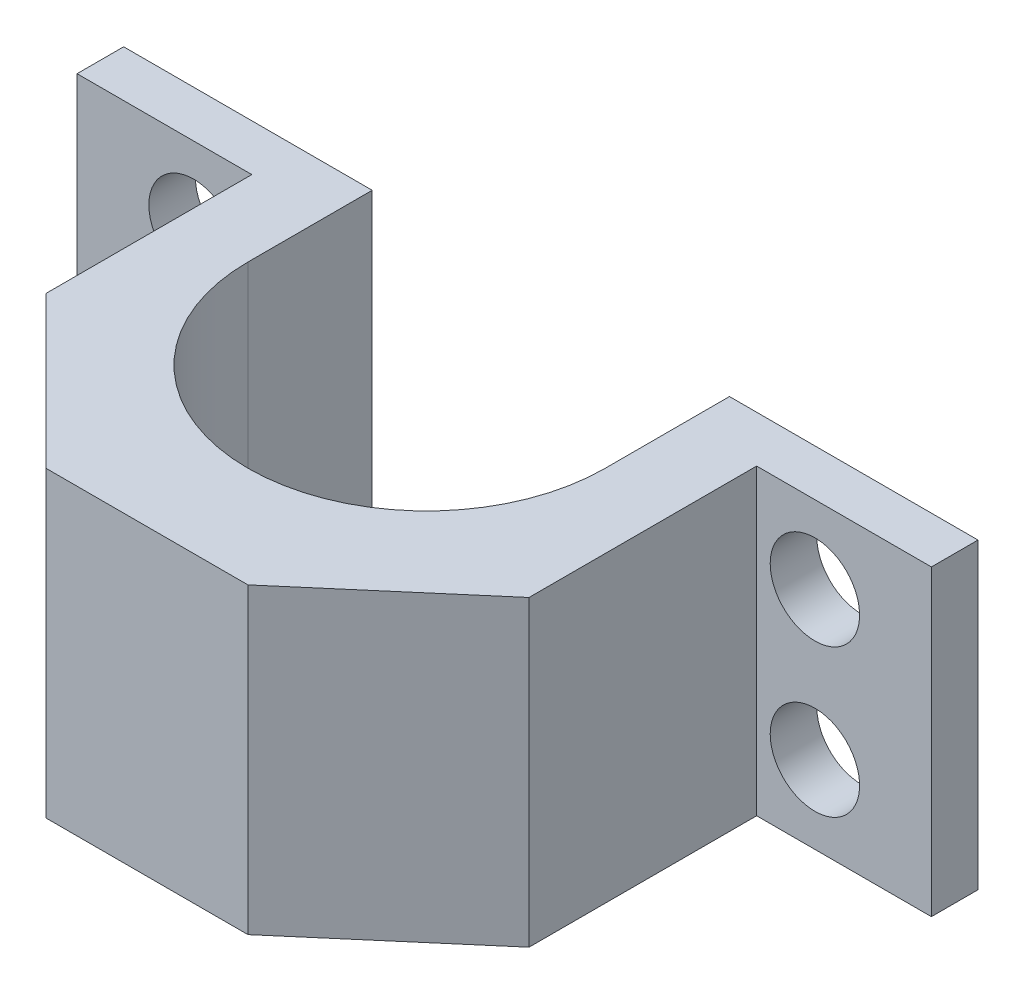
ISO-10303-21;
HEADER;
FILE_DESCRIPTION(('STEP AP214'),'2;1');
FILE_NAME('part.step','',(''),(''),'','','');
FILE_SCHEMA(('AUTOMOTIVE_DESIGN { 1 0 10303 214 1 1 1 1 }'));
ENDSEC;
DATA;
#1=APPLICATION_CONTEXT('core data for automotive mechanical design processes');
#2=APPLICATION_PROTOCOL_DEFINITION('international standard','automotive_design',2000,#1);
#3=PRODUCT_CONTEXT('',#1,'mechanical');
#4=PRODUCT('Part','Part','',(#3));
#5=PRODUCT_RELATED_PRODUCT_CATEGORY('part','',(#4));
#6=PRODUCT_DEFINITION_FORMATION('','',#4);
#7=PRODUCT_DEFINITION_CONTEXT('part definition',#1,'design');
#8=PRODUCT_DEFINITION('design','',#6,#7);
#9=PRODUCT_DEFINITION_SHAPE('','',#8);
#10=(LENGTH_UNIT() NAMED_UNIT(*) SI_UNIT(.MILLI.,.METRE.));
#11=(NAMED_UNIT(*) PLANE_ANGLE_UNIT() SI_UNIT($,.RADIAN.));
#12=(NAMED_UNIT(*) SI_UNIT($,.STERADIAN.) SOLID_ANGLE_UNIT());
#13=UNCERTAINTY_MEASURE_WITH_UNIT(LENGTH_MEASURE(1.E-05),#10,'distance_accuracy_value','');
#14=(GEOMETRIC_REPRESENTATION_CONTEXT(3) GLOBAL_UNCERTAINTY_ASSIGNED_CONTEXT((#13)) GLOBAL_UNIT_ASSIGNED_CONTEXT((#10,
#11,#12)) REPRESENTATION_CONTEXT('',''));
#15=CARTESIAN_POINT('',(0.,0.,0.));
#16=DIRECTION('',(0.,0.,1.));
#17=DIRECTION('',(1.,0.,0.));
#18=AXIS2_PLACEMENT_3D('',#15,#16,#17);
#19=CARTESIAN_POINT('',(32.5,19.5,6.30992988933957));
#20=DIRECTION('',(0.,0.,-1.));
#21=DIRECTION('',(-1.,0.,0.));
#22=AXIS2_PLACEMENT_3D('',#19,#20,#21);
#23=PLANE('',#22);
#24=CARTESIAN_POINT('',(40.,-9.5,6.30992988933957));
#25=DIRECTION('',(0.,0.,-1.));
#26=DIRECTION('',(-1.,0.,0.));
#27=AXIS2_PLACEMENT_3D('',#24,#25,#26);
#28=CIRCLE('',#27,5.7547597151063);
#29=CARTESIAN_POINT('',(34.2452402848937,-9.5,6.30992988933957));
#30=VERTEX_POINT('',#29);
#31=EDGE_CURVE('E180',#30,#30,#28,.T.);
#32=ORIENTED_EDGE('',*,*,#31,.T.);
#33=EDGE_LOOP('',(#32));
#34=FACE_BOUND('',#33,.T.);
#35=CARTESIAN_POINT('',(40.,9.5,6.30992988933957));
#36=DIRECTION('',(0.,0.,-1.));
#37=DIRECTION('',(-1.,0.,0.));
#38=AXIS2_PLACEMENT_3D('',#35,#36,#37);
#39=CIRCLE('',#38,5.7547597151063);
#40=CARTESIAN_POINT('',(34.2452402848937,9.5,6.30992988933957));
#41=VERTEX_POINT('',#40);
#42=EDGE_CURVE('E231',#41,#41,#39,.T.);
#43=ORIENTED_EDGE('',*,*,#42,.T.);
#44=EDGE_LOOP('',(#43));
#45=FACE_BOUND('',#44,.T.);
#46=DIRECTION('',(1.,0.,0.));
#47=VECTOR('',#46,1.);
#48=CARTESIAN_POINT('',(32.5,-19.5,6.30992988933957));
#49=LINE('',#48,#47);
#50=CARTESIAN_POINT('',(32.5,-19.5,6.30992988933957));
#51=VERTEX_POINT('',#50);
#52=CARTESIAN_POINT('',(55.,-19.5,6.30992988933957));
#53=VERTEX_POINT('',#52);
#54=EDGE_CURVE('E175',#51,#53,#49,.T.);
#55=ORIENTED_EDGE('',*,*,#54,.T.);
#56=DIRECTION('',(0.,-1.,0.));
#57=VECTOR('',#56,1.);
#58=CARTESIAN_POINT('',(55.,19.5,6.30992988933957));
#59=LINE('',#58,#57);
#60=CARTESIAN_POINT('',(55.,19.5,6.30992988933957));
#61=VERTEX_POINT('',#60);
#62=EDGE_CURVE('E11',#61,#53,#59,.T.);
#63=ORIENTED_EDGE('',*,*,#62,.F.);
#64=DIRECTION('',(1.,0.,0.));
#65=VECTOR('',#64,1.);
#66=CARTESIAN_POINT('',(32.5,19.5,6.30992988933957));
#67=LINE('',#66,#65);
#68=CARTESIAN_POINT('',(32.5,19.5,6.30992988933957));
#69=VERTEX_POINT('',#68);
#70=EDGE_CURVE('E199',#69,#61,#67,.T.);
#71=ORIENTED_EDGE('',*,*,#70,.F.);
#72=DIRECTION('',(0.,-1.,0.));
#73=VECTOR('',#72,1.);
#74=CARTESIAN_POINT('',(32.5,19.5,6.30992988933957));
#75=LINE('',#74,#73);
#76=EDGE_CURVE('E166',#69,#51,#75,.T.);
#77=ORIENTED_EDGE('',*,*,#76,.T.);
#78=EDGE_LOOP('',(#55,#63,#71,#77));
#79=FACE_BOUND('',#78,.T.);
#80=ADVANCED_FACE('F39',(#34,#45,#79),#23,.F.);
#81=CARTESIAN_POINT('',(55.,19.5,0.309929889339568));
#82=DIRECTION('',(-1.,0.,0.));
#83=DIRECTION('',(0.,0.,1.));
#84=AXIS2_PLACEMENT_3D('',#81,#82,#83);
#85=PLANE('',#84);
#86=DIRECTION('',(0.,0.,-1.));
#87=VECTOR('',#86,1.);
#88=CARTESIAN_POINT('',(55.,-19.5,0.309929889339568));
#89=LINE('',#88,#87);
#90=CARTESIAN_POINT('',(55.,-19.5,0.309929889339568));
#91=VERTEX_POINT('',#90);
#92=EDGE_CURVE('E177',#53,#91,#89,.T.);
#93=ORIENTED_EDGE('',*,*,#92,.T.);
#94=DIRECTION('',(0.,-1.,0.));
#95=VECTOR('',#94,1.);
#96=CARTESIAN_POINT('',(55.,19.5,0.309929889339568));
#97=LINE('',#96,#95);
#98=CARTESIAN_POINT('',(55.,19.5,0.309929889339568));
#99=VERTEX_POINT('',#98);
#100=EDGE_CURVE('E48',#99,#91,#97,.T.);
#101=ORIENTED_EDGE('',*,*,#100,.F.);
#102=DIRECTION('',(0.,0.,-1.));
#103=VECTOR('',#102,1.);
#104=CARTESIAN_POINT('',(55.,19.5,0.309929889339568));
#105=LINE('',#104,#103);
#106=EDGE_CURVE('E120',#61,#99,#105,.T.);
#107=ORIENTED_EDGE('',*,*,#106,.F.);
#108=ORIENTED_EDGE('',*,*,#62,.T.);
#109=EDGE_LOOP('',(#93,#101,#107,#108));
#110=FACE_BOUND('',#109,.T.);
#111=ADVANCED_FACE('F296',(#110),#85,.F.);
#112=CARTESIAN_POINT('',(23.,19.5,0.309929889339568));
#113=DIRECTION('',(0.,0.,1.));
#114=DIRECTION('',(1.,0.,0.));
#115=AXIS2_PLACEMENT_3D('',#112,#113,#114);
#116=PLANE('',#115);
#117=CARTESIAN_POINT('',(40.,-9.5,0.309929889339568));
#118=DIRECTION('',(0.,0.,-1.));
#119=DIRECTION('',(-1.,0.,0.));
#120=AXIS2_PLACEMENT_3D('',#117,#118,#119);
#121=CIRCLE('',#120,5.7547597151063);
#122=CARTESIAN_POINT('',(34.2452402848937,-9.5,0.309929889339568));
#123=VERTEX_POINT('',#122);
#124=EDGE_CURVE('E247',#123,#123,#121,.T.);
#125=ORIENTED_EDGE('',*,*,#124,.F.);
#126=EDGE_LOOP('',(#125));
#127=FACE_BOUND('',#126,.T.);
#128=CARTESIAN_POINT('',(40.,9.5,0.309929889339568));
#129=DIRECTION('',(0.,0.,-1.));
#130=DIRECTION('',(-1.,0.,0.));
#131=AXIS2_PLACEMENT_3D('',#128,#129,#130);
#132=CIRCLE('',#131,5.7547597151063);
#133=CARTESIAN_POINT('',(34.2452402848937,9.5,0.309929889339568));
#134=VERTEX_POINT('',#133);
#135=EDGE_CURVE('E232',#134,#134,#132,.T.);
#136=ORIENTED_EDGE('',*,*,#135,.F.);
#137=EDGE_LOOP('',(#136));
#138=FACE_BOUND('',#137,.T.);
#139=DIRECTION('',(-1.,0.,0.));
#140=VECTOR('',#139,1.);
#141=CARTESIAN_POINT('',(23.,-19.5,0.309929889339568));
#142=LINE('',#141,#140);
#143=CARTESIAN_POINT('',(23.,-19.5,0.309929889339568));
#144=VERTEX_POINT('',#143);
#145=EDGE_CURVE('E179',#91,#144,#142,.T.);
#146=ORIENTED_EDGE('',*,*,#145,.T.);
#147=DIRECTION('',(0.,-1.,0.));
#148=VECTOR('',#147,1.);
#149=CARTESIAN_POINT('',(23.,19.5,0.309929889339568));
#150=LINE('',#149,#148);
#151=CARTESIAN_POINT('',(23.,19.5,0.309929889339568));
#152=VERTEX_POINT('',#151);
#153=EDGE_CURVE('E223',#152,#144,#150,.T.);
#154=ORIENTED_EDGE('',*,*,#153,.F.);
#155=DIRECTION('',(-1.,0.,0.));
#156=VECTOR('',#155,1.);
#157=CARTESIAN_POINT('',(23.,19.5,0.309929889339568));
#158=LINE('',#157,#156);
#159=EDGE_CURVE('E255',#99,#152,#158,.T.);
#160=ORIENTED_EDGE('',*,*,#159,.F.);
#161=ORIENTED_EDGE('',*,*,#100,.T.);
#162=EDGE_LOOP('',(#146,#154,#160,#161));
#163=FACE_BOUND('',#162,.T.);
#164=ADVANCED_FACE('F304',(#127,#138,#163),#116,.F.);
#165=CARTESIAN_POINT('',(23.,19.5,0.309929889339568));
#166=DIRECTION('',(1.,0.,0.));
#167=DIRECTION('',(0.,0.,-1.));
#168=AXIS2_PLACEMENT_3D('',#165,#166,#167);
#169=PLANE('',#168);
#170=DIRECTION('',(0.,0.,1.));
#171=VECTOR('',#170,1.);
#172=CARTESIAN_POINT('',(23.,-19.5,0.309929889339568));
#173=LINE('',#172,#171);
#174=CARTESIAN_POINT('',(23.,-19.5,16.3099298893396));
#175=VERTEX_POINT('',#174);
#176=EDGE_CURVE('E182',#144,#175,#173,.T.);
#177=ORIENTED_EDGE('',*,*,#176,.T.);
#178=DIRECTION('',(0.,-1.,0.));
#179=VECTOR('',#178,1.);
#180=CARTESIAN_POINT('',(23.,19.5,16.3099298893396));
#181=LINE('',#180,#179);
#182=CARTESIAN_POINT('',(23.,19.5,16.3099298893396));
#183=VERTEX_POINT('',#182);
#184=EDGE_CURVE('E225',#183,#175,#181,.T.);
#185=ORIENTED_EDGE('',*,*,#184,.F.);
#186=DIRECTION('',(0.,0.,1.));
#187=VECTOR('',#186,1.);
#188=CARTESIAN_POINT('',(23.,19.5,0.309929889339568));
#189=LINE('',#188,#187);
#190=EDGE_CURVE('E258',#152,#183,#189,.T.);
#191=ORIENTED_EDGE('',*,*,#190,.F.);
#192=ORIENTED_EDGE('',*,*,#153,.T.);
#193=EDGE_LOOP('',(#177,#185,#191,#192));
#194=FACE_BOUND('',#193,.T.);
#195=ADVANCED_FACE('F369',(#194),#169,.F.);
#196=CARTESIAN_POINT('',(0.,19.5,16.3099298893396));
#197=DIRECTION('',(0.,-1.,0.));
#198=DIRECTION('',(0.,0.,-1.));
#199=AXIS2_PLACEMENT_3D('',#196,#197,#198);
#200=CYLINDRICAL_SURFACE('',#199,23.);
#201=CARTESIAN_POINT('',(0.,-19.5,16.3099298893396));
#202=DIRECTION('',(0.,-1.,0.));
#203=DIRECTION('',(0.,0.,1.));
#204=AXIS2_PLACEMENT_3D('',#201,#202,#203);
#205=CIRCLE('',#204,23.);
#206=CARTESIAN_POINT('',(-23.,-19.5,16.3099298893396));
#207=VERTEX_POINT('',#206);
#208=EDGE_CURVE('E181',#175,#207,#205,.T.);
#209=ORIENTED_EDGE('',*,*,#208,.T.);
#210=DIRECTION('',(0.,-1.,0.));
#211=VECTOR('',#210,1.);
#212=CARTESIAN_POINT('',(-23.,19.5,16.3099298893396));
#213=LINE('',#212,#211);
#214=CARTESIAN_POINT('',(-23.,19.5,16.3099298893396));
#215=VERTEX_POINT('',#214);
#216=EDGE_CURVE('E218',#215,#207,#213,.T.);
#217=ORIENTED_EDGE('',*,*,#216,.F.);
#218=CARTESIAN_POINT('',(0.,19.5,16.3099298893396));
#219=DIRECTION('',(0.,-1.,0.));
#220=DIRECTION('',(0.,0.,1.));
#221=AXIS2_PLACEMENT_3D('',#218,#219,#220);
#222=CIRCLE('',#221,23.);
#223=EDGE_CURVE('E256',#183,#215,#222,.T.);
#224=ORIENTED_EDGE('',*,*,#223,.F.);
#225=ORIENTED_EDGE('',*,*,#184,.T.);
#226=EDGE_LOOP('',(#209,#217,#224,#225));
#227=FACE_BOUND('',#226,.T.);
#228=ADVANCED_FACE('F364',(#227),#200,.F.);
#229=CARTESIAN_POINT('',(-23.,19.5,0.309929889339568));
#230=DIRECTION('',(-1.,0.,0.));
#231=DIRECTION('',(0.,0.,1.));
#232=AXIS2_PLACEMENT_3D('',#229,#230,#231);
#233=PLANE('',#232);
#234=DIRECTION('',(0.,0.,-1.));
#235=VECTOR('',#234,1.);
#236=CARTESIAN_POINT('',(-23.,-19.5,0.309929889339568));
#237=LINE('',#236,#235);
#238=CARTESIAN_POINT('',(-23.,-19.5,0.309929889339568));
#239=VERTEX_POINT('',#238);
#240=EDGE_CURVE('E183',#207,#239,#237,.T.);
#241=ORIENTED_EDGE('',*,*,#240,.T.);
#242=DIRECTION('',(0.,-1.,0.));
#243=VECTOR('',#242,1.);
#244=CARTESIAN_POINT('',(-23.,19.5,0.309929889339568));
#245=LINE('',#244,#243);
#246=CARTESIAN_POINT('',(-23.,19.5,0.309929889339568));
#247=VERTEX_POINT('',#246);
#248=EDGE_CURVE('E216',#247,#239,#245,.T.);
#249=ORIENTED_EDGE('',*,*,#248,.F.);
#250=DIRECTION('',(0.,0.,-1.));
#251=VECTOR('',#250,1.);
#252=CARTESIAN_POINT('',(-23.,19.5,0.309929889339568));
#253=LINE('',#252,#251);
#254=EDGE_CURVE('E257',#215,#247,#253,.T.);
#255=ORIENTED_EDGE('',*,*,#254,.F.);
#256=ORIENTED_EDGE('',*,*,#216,.T.);
#257=EDGE_LOOP('',(#241,#249,#255,#256));
#258=FACE_BOUND('',#257,.T.);
#259=ADVANCED_FACE('F340',(#258),#233,.F.);
#260=CARTESIAN_POINT('',(-55.,19.5,0.309929889339568));
#261=DIRECTION('',(0.,0.,1.));
#262=DIRECTION('',(1.,0.,0.));
#263=AXIS2_PLACEMENT_3D('',#260,#261,#262);
#264=PLANE('',#263);
#265=CARTESIAN_POINT('',(-40.,-9.5,0.309929889339568));
#266=DIRECTION('',(0.,0.,-1.));
#267=DIRECTION('',(-1.,0.,0.));
#268=AXIS2_PLACEMENT_3D('',#265,#266,#267);
#269=CIRCLE('',#268,5.7547597151063);
#270=CARTESIAN_POINT('',(-45.7547597151063,-9.5,0.309929889339568));
#271=VERTEX_POINT('',#270);
#272=EDGE_CURVE('E241',#271,#271,#269,.T.);
#273=ORIENTED_EDGE('',*,*,#272,.F.);
#274=EDGE_LOOP('',(#273));
#275=FACE_BOUND('',#274,.T.);
#276=CARTESIAN_POINT('',(-40.,9.5,0.309929889339568));
#277=DIRECTION('',(0.,0.,-1.));
#278=DIRECTION('',(-1.,0.,0.));
#279=AXIS2_PLACEMENT_3D('',#276,#277,#278);
#280=CIRCLE('',#279,5.7547597151063);
#281=CARTESIAN_POINT('',(-45.7547597151063,9.5,0.309929889339568));
#282=VERTEX_POINT('',#281);
#283=EDGE_CURVE('E240',#282,#282,#280,.T.);
#284=ORIENTED_EDGE('',*,*,#283,.F.);
#285=EDGE_LOOP('',(#284));
#286=FACE_BOUND('',#285,.T.);
#287=DIRECTION('',(-1.,0.,0.));
#288=VECTOR('',#287,1.);
#289=CARTESIAN_POINT('',(-55.,-19.5,0.309929889339568));
#290=LINE('',#289,#288);
#291=CARTESIAN_POINT('',(-55.,-19.5,0.309929889339568));
#292=VERTEX_POINT('',#291);
#293=EDGE_CURVE('E186',#239,#292,#290,.T.);
#294=ORIENTED_EDGE('',*,*,#293,.T.);
#295=DIRECTION('',(0.,-1.,0.));
#296=VECTOR('',#295,1.);
#297=CARTESIAN_POINT('',(-55.,19.5,0.309929889339568));
#298=LINE('',#297,#296);
#299=CARTESIAN_POINT('',(-55.,19.5,0.309929889339568));
#300=VERTEX_POINT('',#299);
#301=EDGE_CURVE('E213',#300,#292,#298,.T.);
#302=ORIENTED_EDGE('',*,*,#301,.F.);
#303=DIRECTION('',(-1.,0.,0.));
#304=VECTOR('',#303,1.);
#305=CARTESIAN_POINT('',(-55.,19.5,0.309929889339568));
#306=LINE('',#305,#304);
#307=EDGE_CURVE('E265',#247,#300,#306,.T.);
#308=ORIENTED_EDGE('',*,*,#307,.F.);
#309=ORIENTED_EDGE('',*,*,#248,.T.);
#310=EDGE_LOOP('',(#294,#302,#308,#309));
#311=FACE_BOUND('',#310,.T.);
#312=ADVANCED_FACE('F331',(#275,#286,#311),#264,.F.);
#313=CARTESIAN_POINT('',(-55.,19.5,0.309929889339568));
#314=DIRECTION('',(1.,0.,0.));
#315=DIRECTION('',(0.,0.,-1.));
#316=AXIS2_PLACEMENT_3D('',#313,#314,#315);
#317=PLANE('',#316);
#318=DIRECTION('',(0.,0.,1.));
#319=VECTOR('',#318,1.);
#320=CARTESIAN_POINT('',(-55.,-19.5,0.309929889339568));
#321=LINE('',#320,#319);
#322=CARTESIAN_POINT('',(-55.,-19.5,6.30992988933957));
#323=VERTEX_POINT('',#322);
#324=EDGE_CURVE('E188',#292,#323,#321,.T.);
#325=ORIENTED_EDGE('',*,*,#324,.T.);
#326=DIRECTION('',(0.,-1.,0.));
#327=VECTOR('',#326,1.);
#328=CARTESIAN_POINT('',(-55.,19.5,6.30992988933957));
#329=LINE('',#328,#327);
#330=CARTESIAN_POINT('',(-55.,19.5,6.30992988933957));
#331=VERTEX_POINT('',#330);
#332=EDGE_CURVE('E209',#331,#323,#329,.T.);
#333=ORIENTED_EDGE('',*,*,#332,.F.);
#334=DIRECTION('',(0.,0.,1.));
#335=VECTOR('',#334,1.);
#336=CARTESIAN_POINT('',(-55.,19.5,0.309929889339568));
#337=LINE('',#336,#335);
#338=EDGE_CURVE('E262',#300,#331,#337,.T.);
#339=ORIENTED_EDGE('',*,*,#338,.F.);
#340=ORIENTED_EDGE('',*,*,#301,.T.);
#341=EDGE_LOOP('',(#325,#333,#339,#340));
#342=FACE_BOUND('',#341,.T.);
#343=ADVANCED_FACE('F336',(#342),#317,.F.);
#344=CARTESIAN_POINT('',(-55.,19.5,6.30992988933957));
#345=DIRECTION('',(0.,0.,-1.));
#346=DIRECTION('',(-1.,0.,0.));
#347=AXIS2_PLACEMENT_3D('',#344,#345,#346);
#348=PLANE('',#347);
#349=CARTESIAN_POINT('',(-40.,-9.5,6.30992988933957));
#350=DIRECTION('',(0.,0.,-1.));
#351=DIRECTION('',(-1.,0.,0.));
#352=AXIS2_PLACEMENT_3D('',#349,#350,#351);
#353=CIRCLE('',#352,5.7547597151063);
#354=CARTESIAN_POINT('',(-45.7547597151063,-9.5,6.30992988933957));
#355=VERTEX_POINT('',#354);
#356=EDGE_CURVE('E45',#355,#355,#353,.T.);
#357=ORIENTED_EDGE('',*,*,#356,.T.);
#358=EDGE_LOOP('',(#357));
#359=FACE_BOUND('',#358,.T.);
#360=CARTESIAN_POINT('',(-40.,9.5,6.30992988933957));
#361=DIRECTION('',(0.,0.,-1.));
#362=DIRECTION('',(-1.,0.,0.));
#363=AXIS2_PLACEMENT_3D('',#360,#361,#362);
#364=CIRCLE('',#363,5.7547597151063);
#365=CARTESIAN_POINT('',(-45.7547597151063,9.5,6.30992988933957));
#366=VERTEX_POINT('',#365);
#367=EDGE_CURVE('E228',#366,#366,#364,.T.);
#368=ORIENTED_EDGE('',*,*,#367,.T.);
#369=EDGE_LOOP('',(#368));
#370=FACE_BOUND('',#369,.T.);
#371=DIRECTION('',(1.,0.,0.));
#372=VECTOR('',#371,1.);
#373=CARTESIAN_POINT('',(-55.,-19.5,6.30992988933957));
#374=LINE('',#373,#372);
#375=CARTESIAN_POINT('',(-32.5,-19.5,6.30992988933957));
#376=VERTEX_POINT('',#375);
#377=EDGE_CURVE('E192',#323,#376,#374,.T.);
#378=ORIENTED_EDGE('',*,*,#377,.T.);
#379=DIRECTION('',(0.,-1.,0.));
#380=VECTOR('',#379,1.);
#381=CARTESIAN_POINT('',(-32.5,19.5,6.30992988933957));
#382=LINE('',#381,#380);
#383=CARTESIAN_POINT('',(-32.5,19.5,6.30992988933957));
#384=VERTEX_POINT('',#383);
#385=EDGE_CURVE('E210',#384,#376,#382,.T.);
#386=ORIENTED_EDGE('',*,*,#385,.F.);
#387=DIRECTION('',(1.,0.,0.));
#388=VECTOR('',#387,1.);
#389=CARTESIAN_POINT('',(-55.,19.5,6.30992988933957));
#390=LINE('',#389,#388);
#391=EDGE_CURVE('E266',#331,#384,#390,.T.);
#392=ORIENTED_EDGE('',*,*,#391,.F.);
#393=ORIENTED_EDGE('',*,*,#332,.T.);
#394=EDGE_LOOP('',(#378,#386,#392,#393));
#395=FACE_BOUND('',#394,.T.);
#396=ADVANCED_FACE('F351',(#359,#370,#395),#348,.F.);
#397=CARTESIAN_POINT('',(-32.5,19.5,6.30992988933957));
#398=DIRECTION('',(1.,0.,0.));
#399=DIRECTION('',(0.,0.,-1.));
#400=AXIS2_PLACEMENT_3D('',#397,#398,#399);
#401=PLANE('',#400);
#402=DIRECTION('',(0.,0.,1.));
#403=VECTOR('',#402,1.);
#404=CARTESIAN_POINT('',(-32.5,-19.5,6.30992988933957));
#405=LINE('',#404,#403);
#406=CARTESIAN_POINT('',(-32.5,-19.5,32.8099298893396));
#407=VERTEX_POINT('',#406);
#408=EDGE_CURVE('E193',#376,#407,#405,.T.);
#409=ORIENTED_EDGE('',*,*,#408,.T.);
#410=DIRECTION('',(0.,-1.,0.));
#411=VECTOR('',#410,1.);
#412=CARTESIAN_POINT('',(-32.5,19.5,32.8099298893396));
#413=LINE('',#412,#411);
#414=CARTESIAN_POINT('',(-32.5,19.5,32.8099298893396));
#415=VERTEX_POINT('',#414);
#416=EDGE_CURVE('E204',#415,#407,#413,.T.);
#417=ORIENTED_EDGE('',*,*,#416,.F.);
#418=DIRECTION('',(0.,0.,1.));
#419=VECTOR('',#418,1.);
#420=CARTESIAN_POINT('',(-32.5,19.5,6.30992988933957));
#421=LINE('',#420,#419);
#422=EDGE_CURVE('E268',#384,#415,#421,.T.);
#423=ORIENTED_EDGE('',*,*,#422,.F.);
#424=ORIENTED_EDGE('',*,*,#385,.T.);
#425=EDGE_LOOP('',(#409,#417,#423,#424));
#426=FACE_BOUND('',#425,.T.);
#427=ADVANCED_FACE('F273',(#426),#401,.F.);
#428=CARTESIAN_POINT('',(-32.5,19.5,32.8099298893396));
#429=DIRECTION('',(0.707106781186548,0.,-0.707106781186547));
#430=DIRECTION('',(-0.707106781186547,0.,-0.707106781186548));
#431=AXIS2_PLACEMENT_3D('',#428,#429,#430);
#432=PLANE('',#431);
#433=DIRECTION('',(0.707106781186547,0.,0.707106781186548));
#434=VECTOR('',#433,1.);
#435=CARTESIAN_POINT('',(-32.5,-19.5,32.8099298893396));
#436=LINE('',#435,#434);
#437=CARTESIAN_POINT('',(-13.,-19.5,52.3099298893396));
#438=VERTEX_POINT('',#437);
#439=EDGE_CURVE('E191',#407,#438,#436,.T.);
#440=ORIENTED_EDGE('',*,*,#439,.T.);
#441=DIRECTION('',(0.,-1.,0.));
#442=VECTOR('',#441,1.);
#443=CARTESIAN_POINT('',(-13.,19.5,52.3099298893396));
#444=LINE('',#443,#442);
#445=CARTESIAN_POINT('',(-13.,19.5,52.3099298893396));
#446=VERTEX_POINT('',#445);
#447=EDGE_CURVE('E163',#446,#438,#444,.T.);
#448=ORIENTED_EDGE('',*,*,#447,.F.);
#449=DIRECTION('',(0.707106781186547,0.,0.707106781186548));
#450=VECTOR('',#449,1.);
#451=CARTESIAN_POINT('',(-32.5,19.5,32.8099298893396));
#452=LINE('',#451,#450);
#453=EDGE_CURVE('E154',#415,#446,#452,.T.);
#454=ORIENTED_EDGE('',*,*,#453,.F.);
#455=ORIENTED_EDGE('',*,*,#416,.T.);
#456=EDGE_LOOP('',(#440,#448,#454,#455));
#457=FACE_BOUND('',#456,.T.);
#458=ADVANCED_FACE('F279',(#457),#432,.F.);
#459=CARTESIAN_POINT('',(-13.,19.5,52.3099298893396));
#460=DIRECTION('',(0.,0.,-1.));
#461=DIRECTION('',(-1.,0.,0.));
#462=AXIS2_PLACEMENT_3D('',#459,#460,#461);
#463=PLANE('',#462);
#464=DIRECTION('',(1.,0.,0.));
#465=VECTOR('',#464,1.);
#466=CARTESIAN_POINT('',(-13.,-19.5,52.3099298893396));
#467=LINE('',#466,#465);
#468=CARTESIAN_POINT('',(13.,-19.5,52.3099298893396));
#469=VERTEX_POINT('',#468);
#470=EDGE_CURVE('E162',#438,#469,#467,.T.);
#471=ORIENTED_EDGE('',*,*,#470,.T.);
#472=DIRECTION('',(0.,-1.,0.));
#473=VECTOR('',#472,1.);
#474=CARTESIAN_POINT('',(13.,19.5,52.3099298893396));
#475=LINE('',#474,#473);
#476=CARTESIAN_POINT('',(13.,19.5,52.3099298893396));
#477=VERTEX_POINT('',#476);
#478=EDGE_CURVE('E159',#477,#469,#475,.T.);
#479=ORIENTED_EDGE('',*,*,#478,.F.);
#480=DIRECTION('',(1.,0.,0.));
#481=VECTOR('',#480,1.);
#482=CARTESIAN_POINT('',(-13.,19.5,52.3099298893396));
#483=LINE('',#482,#481);
#484=EDGE_CURVE('E149',#446,#477,#483,.T.);
#485=ORIENTED_EDGE('',*,*,#484,.F.);
#486=ORIENTED_EDGE('',*,*,#447,.T.);
#487=EDGE_LOOP('',(#471,#479,#485,#486));
#488=FACE_BOUND('',#487,.T.);
#489=ADVANCED_FACE('F161',(#488),#463,.F.);
#490=CARTESIAN_POINT('',(13.,19.5,52.3099298893396));
#491=DIRECTION('',(-0.650261007779441,0.,-0.759710880375993));
#492=DIRECTION('',(-0.759710880375993,0.,0.650261007779441));
#493=AXIS2_PLACEMENT_3D('',#490,#491,#492);
#494=PLANE('',#493);
#495=DIRECTION('',(0.759710880375993,0.,-0.650261007779441));
#496=VECTOR('',#495,1.);
#497=CARTESIAN_POINT('',(13.,-19.5,52.3099298893396));
#498=LINE('',#497,#496);
#499=CARTESIAN_POINT('',(32.5,-19.5,35.6192519232382));
#500=VERTEX_POINT('',#499);
#501=EDGE_CURVE('E102',#469,#500,#498,.T.);
#502=ORIENTED_EDGE('',*,*,#501,.T.);
#503=DIRECTION('',(0.,-1.,0.));
#504=VECTOR('',#503,1.);
#505=CARTESIAN_POINT('',(32.5,19.5,35.6192519232382));
#506=LINE('',#505,#504);
#507=CARTESIAN_POINT('',(32.5,19.5,35.6192519232382));
#508=VERTEX_POINT('',#507);
#509=EDGE_CURVE('E164',#508,#500,#506,.T.);
#510=ORIENTED_EDGE('',*,*,#509,.F.);
#511=DIRECTION('',(0.759710880375993,0.,-0.650261007779441));
#512=VECTOR('',#511,1.);
#513=CARTESIAN_POINT('',(13.,19.5,52.3099298893396));
#514=LINE('',#513,#512);
#515=EDGE_CURVE('E153',#477,#508,#514,.T.);
#516=ORIENTED_EDGE('',*,*,#515,.F.);
#517=ORIENTED_EDGE('',*,*,#478,.T.);
#518=EDGE_LOOP('',(#502,#510,#516,#517));
#519=FACE_BOUND('',#518,.T.);
#520=ADVANCED_FACE('F170',(#519),#494,.F.);
#521=CARTESIAN_POINT('',(32.5,19.5,35.6192519232382));
#522=DIRECTION('',(-1.,0.,0.));
#523=DIRECTION('',(0.,0.,1.));
#524=AXIS2_PLACEMENT_3D('',#521,#522,#523);
#525=PLANE('',#524);
#526=DIRECTION('',(0.,0.,-1.));
#527=VECTOR('',#526,1.);
#528=CARTESIAN_POINT('',(32.5,-19.5,35.6192519232382));
#529=LINE('',#528,#527);
#530=EDGE_CURVE('E109',#500,#51,#529,.T.);
#531=ORIENTED_EDGE('',*,*,#530,.T.);
#532=ORIENTED_EDGE('',*,*,#76,.F.);
#533=DIRECTION('',(0.,0.,-1.));
#534=VECTOR('',#533,1.);
#535=CARTESIAN_POINT('',(32.5,19.5,35.6192519232382));
#536=LINE('',#535,#534);
#537=EDGE_CURVE('E60',#508,#69,#536,.T.);
#538=ORIENTED_EDGE('',*,*,#537,.F.);
#539=ORIENTED_EDGE('',*,*,#509,.T.);
#540=EDGE_LOOP('',(#531,#532,#538,#539));
#541=FACE_BOUND('',#540,.T.);
#542=ADVANCED_FACE('F287',(#541),#525,.F.);
#543=CARTESIAN_POINT('',(0.,19.5,16.3099298893396));
#544=DIRECTION('',(0.,1.,0.));
#545=DIRECTION('',(0.,0.,1.));
#546=AXIS2_PLACEMENT_3D('',#543,#544,#545);
#547=PLANE('',#546);
#548=ORIENTED_EDGE('',*,*,#70,.T.);
#549=ORIENTED_EDGE('',*,*,#106,.T.);
#550=ORIENTED_EDGE('',*,*,#159,.T.);
#551=ORIENTED_EDGE('',*,*,#190,.T.);
#552=ORIENTED_EDGE('',*,*,#223,.T.);
#553=ORIENTED_EDGE('',*,*,#254,.T.);
#554=ORIENTED_EDGE('',*,*,#307,.T.);
#555=ORIENTED_EDGE('',*,*,#338,.T.);
#556=ORIENTED_EDGE('',*,*,#391,.T.);
#557=ORIENTED_EDGE('',*,*,#422,.T.);
#558=ORIENTED_EDGE('',*,*,#453,.T.);
#559=ORIENTED_EDGE('',*,*,#484,.T.);
#560=ORIENTED_EDGE('',*,*,#515,.T.);
#561=ORIENTED_EDGE('',*,*,#537,.T.);
#562=EDGE_LOOP('',(#548,#549,#550,#551,#552,#553,#554,#555,#556,#557,#558,#559,#560,#561));
#563=FACE_BOUND('',#562,.T.);
#564=ADVANCED_FACE('F151',(#563),#547,.T.);
#565=CARTESIAN_POINT('',(0.,-19.5,16.3099298893396));
#566=DIRECTION('',(0.,1.,0.));
#567=DIRECTION('',(0.,0.,1.));
#568=AXIS2_PLACEMENT_3D('',#565,#566,#567);
#569=PLANE('',#568);
#570=ORIENTED_EDGE('',*,*,#54,.F.);
#571=ORIENTED_EDGE('',*,*,#530,.F.);
#572=ORIENTED_EDGE('',*,*,#501,.F.);
#573=ORIENTED_EDGE('',*,*,#470,.F.);
#574=ORIENTED_EDGE('',*,*,#439,.F.);
#575=ORIENTED_EDGE('',*,*,#408,.F.);
#576=ORIENTED_EDGE('',*,*,#377,.F.);
#577=ORIENTED_EDGE('',*,*,#324,.F.);
#578=ORIENTED_EDGE('',*,*,#293,.F.);
#579=ORIENTED_EDGE('',*,*,#240,.F.);
#580=ORIENTED_EDGE('',*,*,#208,.F.);
#581=ORIENTED_EDGE('',*,*,#176,.F.);
#582=ORIENTED_EDGE('',*,*,#145,.F.);
#583=ORIENTED_EDGE('',*,*,#92,.F.);
#584=EDGE_LOOP('',(#570,#571,#572,#573,#574,#575,#576,#577,#578,#579,#580,#581,#582,#583));
#585=FACE_BOUND('',#584,.T.);
#586=ADVANCED_FACE('F284',(#585),#569,.F.);
#587=CARTESIAN_POINT('',(-40.,9.5,39.3099298893396));
#588=DIRECTION('',(0.,0.,-1.));
#589=DIRECTION('',(-1.,0.,0.));
#590=AXIS2_PLACEMENT_3D('',#587,#588,#589);
#591=CYLINDRICAL_SURFACE('',#590,5.7547597151063);
#592=ORIENTED_EDGE('',*,*,#283,.T.);
#593=EDGE_LOOP('',(#592));
#594=FACE_BOUND('',#593,.T.);
#595=ORIENTED_EDGE('',*,*,#367,.F.);
#596=EDGE_LOOP('',(#595));
#597=FACE_BOUND('',#596,.T.);
#598=ADVANCED_FACE('F319',(#594,#597),#591,.F.);
#599=CARTESIAN_POINT('',(-40.,-9.5,39.3099298893396));
#600=DIRECTION('',(0.,0.,-1.));
#601=DIRECTION('',(-1.,0.,0.));
#602=AXIS2_PLACEMENT_3D('',#599,#600,#601);
#603=CYLINDRICAL_SURFACE('',#602,5.7547597151063);
#604=ORIENTED_EDGE('',*,*,#272,.T.);
#605=EDGE_LOOP('',(#604));
#606=FACE_BOUND('',#605,.T.);
#607=ORIENTED_EDGE('',*,*,#356,.F.);
#608=EDGE_LOOP('',(#607));
#609=FACE_BOUND('',#608,.T.);
#610=ADVANCED_FACE('F315',(#606,#609),#603,.F.);
#611=CARTESIAN_POINT('',(40.,9.5,39.3099298893396));
#612=DIRECTION('',(0.,0.,-1.));
#613=DIRECTION('',(-1.,0.,0.));
#614=AXIS2_PLACEMENT_3D('',#611,#612,#613);
#615=CYLINDRICAL_SURFACE('',#614,5.7547597151063);
#616=ORIENTED_EDGE('',*,*,#135,.T.);
#617=EDGE_LOOP('',(#616));
#618=FACE_BOUND('',#617,.T.);
#619=ORIENTED_EDGE('',*,*,#42,.F.);
#620=EDGE_LOOP('',(#619));
#621=FACE_BOUND('',#620,.T.);
#622=ADVANCED_FACE('F310',(#618,#621),#615,.F.);
#623=CARTESIAN_POINT('',(40.,-9.5,39.3099298893396));
#624=DIRECTION('',(0.,0.,-1.));
#625=DIRECTION('',(-1.,0.,0.));
#626=AXIS2_PLACEMENT_3D('',#623,#624,#625);
#627=CYLINDRICAL_SURFACE('',#626,5.7547597151063);
#628=ORIENTED_EDGE('',*,*,#124,.T.);
#629=EDGE_LOOP('',(#628));
#630=FACE_BOUND('',#629,.T.);
#631=ORIENTED_EDGE('',*,*,#31,.F.);
#632=EDGE_LOOP('',(#631));
#633=FACE_BOUND('',#632,.T.);
#634=ADVANCED_FACE('F313',(#630,#633),#627,.F.);
#635=CLOSED_SHELL('',(#80,#111,#164,#195,#228,#259,#312,#343,#396,#427,#458,#489,#520,#542,#564,
#586,#598,#610,#622,#634));
#636=MANIFOLD_SOLID_BREP('B2',#635);
#637=ADVANCED_BREP_SHAPE_REPRESENTATION('',(#18,#636),#14);
#638=SHAPE_DEFINITION_REPRESENTATION(#9,#637);
ENDSEC;
END-ISO-10303-21;
